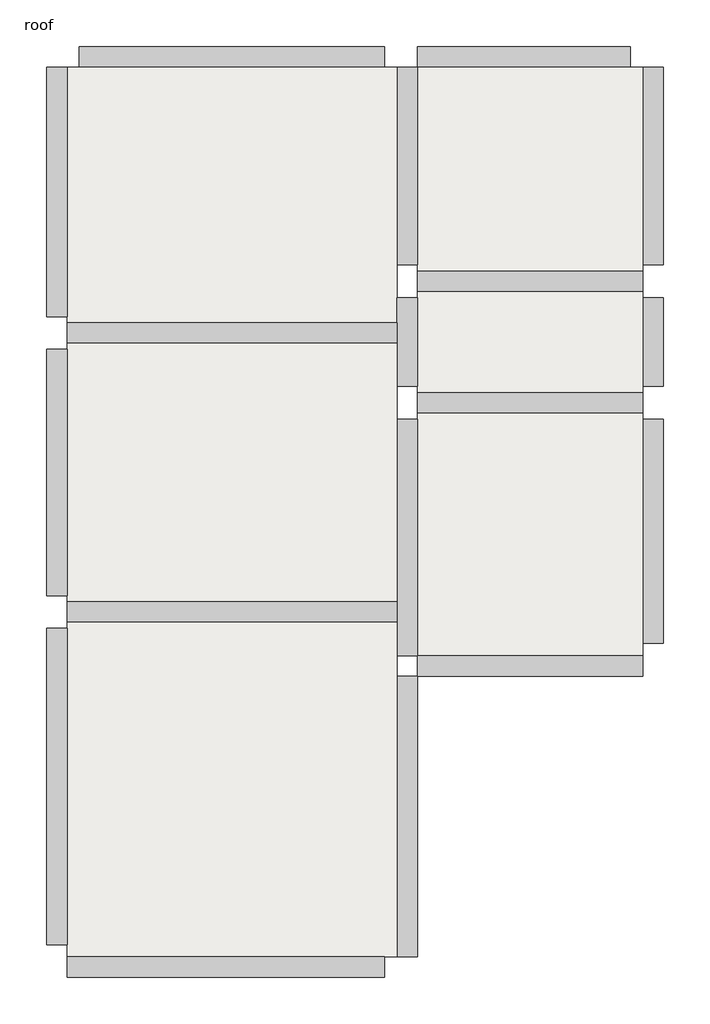
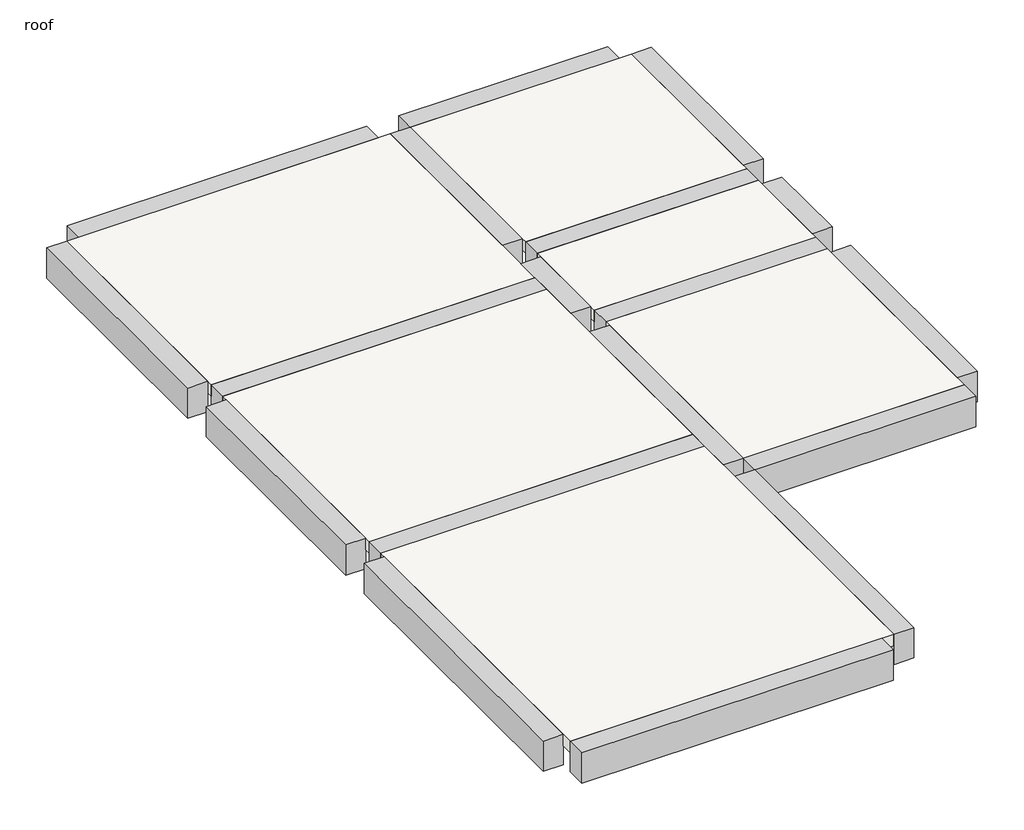
# One storey: 18 beams, 6 slabs.
"""IFC4 building model written with IfcOpenShell, lengths in millimetres."""

from ifc_helpers import new_model, si_unit, frame, origin, place, context, project, spatial, polyline, outline, extrude, faceted_brep, element, save

model = new_model("IFC4")

# Units and contexts
model_context = context("Model", 3, world=origin())
ifc_project = project(units=[si_unit("LENGTHUNIT", "METRE", prefix="MILLI")], contexts=[model_context])

# Site, building, storey
site = spatial("IfcSite", under=ifc_project)
building = spatial("IfcBuilding", under=site)
storey = spatial("IfcBuildingStorey", under=building, Name="roof", Elevation=6400.8)

# Beams
placement = place(None, origin())
element("IfcBeam", 1, ObjectType="Concrete-Rectangular Beam : BEAM", at=placement, inside=storey, context=model_context, shape_type="SweptSolid", body=[
    extrude(outline(polyline([(-12336.5990423, 3901.2699494), (-12082.5990423, 3901.2699494), (-12082.5990423, -16.6800506), (-12336.5990423, -16.6800506), (-12336.5990423, 3901.2699494)])), frame((0.0, 0.0, 5994.4), z_axis=(0.0, 0.0, 1.0), x_axis=(1.0, 0.0, 0.0)), (0.0, 0.0, 1.0), 406.4),
])
element("IfcBeam", 2, ObjectType="Concrete-Rectangular Beam : BEAM", at=placement, inside=storey, context=model_context, shape_type="SweptSolid", body=[
    extrude(outline(polyline([(-12336.5990423, 7355.6699494), (-12082.5990423, 7355.6699494), (-12082.5990423, 4307.6699494), (-12336.5990423, 4307.6699494), (-12336.5990423, 7355.6699494)])), frame((0.0, 0.0, 5994.4), z_axis=(0.0, 0.0, 1.0), x_axis=(1.0, 0.0, 0.0)), (0.0, 0.0, 1.0), 406.4),
])
element("IfcBeam", 3, ObjectType="Concrete-Rectangular Beam : BEAM", at=placement, inside=storey, context=model_context, shape_type="Brep", body=[
    faceted_brep([(-12082.5990423, 10854.5199494, 6400.8), (-12336.5990423, 10854.5199494, 6400.8), (-12336.5990423, 7762.0699494, 6400.8), (-12082.5990423, 7762.0699494, 6400.8), (-12082.5990423, 10854.5199494, 5994.4), (-12082.5990423, 10854.5199494, 6248.4), (-12082.5990423, 7762.0699494, 5994.4), (-12336.5990423, 10854.5199494, 5994.4), (-12336.5990423, 7762.0699494, 5994.4)], [[[0, 1, 2, 3]], [[4, 5, 0, 3, 6]], [[7, 4, 6, 8]], [[1, 7, 8, 2]], [[1, 0, 5, 4, 7]], [[3, 2, 8, 6]]]),
])
element("IfcBeam", 4, ObjectType="Concrete-Rectangular Beam : BEAM", at=placement, inside=storey, context=model_context, shape_type="SweptSolid", body=[
    extrude(outline(polyline([(-11930.1990423, 10854.5199494), (-11930.1990423, 11108.5199494), (-8145.5990423, 11108.5199494), (-8145.5990423, 10854.5199494), (-11930.1990423, 10854.5199494)])), frame((0.0, 0.0, 5994.4), z_axis=(0.0, 0.0, 1.0), x_axis=(1.0, 0.0, 0.0)), (0.0, 0.0, 1.0), 406.4),
])
element("IfcBeam", 5, ObjectType="Concrete-Rectangular Beam : BEAM", at=placement, inside=storey, context=model_context, shape_type="Brep", body=[
    faceted_brep([(-7739.1990423, 11108.5199494, 6400.8), (-7739.1990423, 10854.5199494, 6400.8), (-5097.5990423, 10854.5199494, 6400.8), (-5097.5990423, 11108.5199494, 6400.8), (-7739.1990423, 10854.5199494, 6248.4), (-7739.1990423, 10854.5199494, 5994.4), (-5097.5990423, 10854.5199494, 5994.4), (-7739.1990423, 11108.5199494, 5994.4), (-5097.5990423, 11108.5199494, 5994.4)], [[[0, 1, 2, 3]], [[1, 4, 5, 6, 2]], [[5, 7, 8, 6]], [[7, 0, 3, 8]], [[5, 4, 1, 0, 7]], [[3, 2, 6, 8]]]),
])
element("IfcBeam", 6, ObjectType="Concrete-Rectangular Beam : BEAM", at=placement, inside=storey, context=model_context, shape_type="Brep", body=[
    faceted_brep([(-4691.1990423, 10854.5199494, 6400.8), (-4945.1990423, 10854.5199494, 6400.8), (-4945.1990423, 8403.4199494, 6400.8), (-4691.1990423, 8403.4199494, 6400.8), (-4691.1990423, 10854.5199494, 5994.4), (-4691.1990423, 8403.4199494, 5994.4), (-4945.1990423, 10854.5199494, 5994.4), (-4945.1990423, 8403.4199494, 5994.4), (-4945.1990423, 10854.5199494, 6248.4)], [[[0, 1, 2, 3]], [[4, 0, 3, 5]], [[6, 4, 5, 7]], [[1, 8, 6, 7, 2]], [[6, 8, 1, 0, 4]], [[3, 2, 7, 5]]]),
])
element("IfcBeam", 7, ObjectType="Concrete-Rectangular Beam : BEAM", at=placement, inside=storey, context=model_context, shape_type="SweptSolid", body=[
    extrude(outline(polyline([(-4945.1990423, 7997.0199494), (-4691.1990423, 7997.0199494), (-4691.1990423, 6898.4699494), (-4945.1990423, 6898.4699494), (-4945.1990423, 7997.0199494)])), frame((0.0, 0.0, 5994.4), z_axis=(0.0, 0.0, 1.0), x_axis=(1.0, 0.0, 0.0)), (0.0, 0.0, 1.0), 406.4),
])
element("IfcBeam", 8, ObjectType="Concrete-Rectangular Beam : BEAM", at=placement, inside=storey, context=model_context, shape_type="SweptSolid", body=[
    extrude(outline(polyline([(-4691.1990423, 3717.1199494), (-4945.1990423, 3717.1199494), (-4945.1990423, 6492.0699494), (-4691.1990423, 6492.0699494), (-4691.1990423, 3717.1199494)])), frame((0.0, 0.0, 5994.4), z_axis=(0.0, 0.0, 1.0), x_axis=(1.0, 0.0, 0.0)), (0.0, 0.0, 1.0), 406.4),
])
element("IfcBeam", 9, ObjectType="Concrete-Rectangular Beam : BEAM", at=placement, inside=storey, context=model_context, shape_type="Brep", body=[
    faceted_brep([(-4945.1990423, 3310.7199494, 6400.8), (-4945.1990423, 3564.7199494, 6400.8), (-7739.1990423, 3564.7199494, 6400.8), (-7739.1990423, 3310.7199494, 6400.8), (-4945.1990423, 3564.7199494, 6248.4), (-4945.1990423, 3564.7199494, 5994.4), (-7739.1990423, 3564.7199494, 5994.4), (-7739.1990423, 3564.7199494, 6248.4), (-4945.1990423, 3310.7199494, 5994.4), (-7739.1990423, 3310.7199494, 5994.4)], [[[0, 1, 2, 3]], [[1, 4, 5, 6, 7, 2]], [[5, 8, 9, 6]], [[3, 9, 8, 0]], [[0, 8, 5, 4, 1]], [[3, 2, 7, 6, 9]]]),
])
element("IfcBeam", 10, ObjectType="Concrete-Rectangular Beam : BEAM", at=placement, inside=storey, context=model_context, shape_type="Brep", body=[
    faceted_brep([(-7993.1990423, 3564.7199494, 6400.8), (-7739.1990423, 3564.7199494, 6400.8), (-7739.1990423, 6492.0699494, 6400.8), (-7993.1990423, 6492.0699494, 6400.8), (-7993.1990423, 4231.4699494, 6400.8), (-7993.1990423, 3977.4699494, 6400.8), (-7993.1990423, 3564.7199494, 5994.4), (-7993.1990423, 6492.0699494, 5994.4), (-7993.1990423, 4231.4699494, 5994.4), (-7993.1990423, 3977.4699494, 5994.4), (-7739.1990423, 3564.7199494, 5994.4), (-7739.1990423, 6492.0699494, 5994.4), (-7739.1990423, 3564.7199494, 6248.4)], [[[0, 1, 2, 3, 4, 5]], [[6, 0, 5, 4, 3, 7, 8, 9]], [[10, 6, 9, 8, 7, 11]], [[1, 12, 10, 11, 2]], [[10, 12, 1, 0, 6]], [[3, 2, 11, 7]]]),
])
element("IfcBeam", 11, ObjectType="Concrete-Rectangular Beam : BEAM", at=placement, inside=storey, context=model_context, shape_type="Brep", body=[
    faceted_brep([(-7993.1990423, 6898.4699494, 6400.8), (-7739.1990423, 6898.4699494, 6400.8), (-7739.1990423, 7997.0199494, 6400.8), (-7993.1990423, 7997.0199494, 6400.8), (-7993.1990423, 7685.8699494, 6400.8), (-7993.1990423, 7431.8699494, 6400.8), (-7739.1990423, 6898.4699494, 5994.4), (-7739.1990423, 7997.0199494, 5994.4), (-7993.1990423, 6898.4699494, 5994.4), (-7993.1990423, 7431.8699494, 5994.4), (-7993.1990423, 7685.8699494, 5994.4), (-7993.1990423, 7997.0199494, 5994.4)], [[[0, 1, 2, 3, 4, 5]], [[1, 6, 7, 2]], [[6, 8, 9, 10, 11, 7]], [[8, 0, 5, 4, 3, 11, 10, 9]], [[1, 0, 8, 6]], [[3, 2, 7, 11]]]),
])
element("IfcBeam", 12, ObjectType="Concrete-Rectangular Beam : BEAM", at=placement, inside=storey, context=model_context, shape_type="Brep", body=[
    faceted_brep([(-7739.1990423, 10854.5199494, 6400.8), (-7993.1990423, 10854.5199494, 6400.8), (-7993.1990423, 8403.4199494, 6400.8), (-7739.1990423, 8403.4199494, 6400.8), (-7739.1990423, 10854.5199494, 5994.4), (-7739.1990423, 10854.5199494, 6248.4), (-7739.1990423, 8403.4199494, 5994.4), (-7993.1990423, 10854.5199494, 5994.4), (-7993.1990423, 8403.4199494, 5994.4), (-7993.1990423, 10854.5199494, 6248.4)], [[[0, 1, 2, 3]], [[4, 5, 0, 3, 6]], [[7, 4, 6, 8]], [[1, 9, 7, 8, 2]], [[7, 9, 1, 0, 5, 4]], [[3, 2, 8, 6]]]),
])
element("IfcBeam", 13, ObjectType="Concrete-Rectangular Beam : BEAM", at=placement, inside=storey, context=model_context, shape_type="Brep", body=[
    faceted_brep([(-7739.1990423, 3310.7199494, 6400.8), (-7993.1990423, 3310.7199494, 6400.8), (-7993.1990423, -169.0800506, 6400.8), (-7739.1990423, -169.0800506, 6400.8), (-7993.1990423, 3310.7199494, 5994.4), (-7993.1990423, -169.0800506, 5994.4), (-7993.1990423, -169.0800506, 6248.4), (-7739.1990423, 3310.7199494, 5994.4), (-7739.1990423, -169.0800506, 5994.4)], [[[0, 1, 2, 3]], [[1, 4, 5, 6, 2]], [[4, 7, 8, 5]], [[7, 0, 3, 8]], [[0, 7, 4, 1]], [[3, 2, 6, 5, 8]]]),
])
element("IfcBeam", 14, ObjectType="Concrete-Rectangular Beam : BEAM", at=placement, inside=storey, context=model_context, shape_type="Brep", body=[
    faceted_brep([(-12082.5990423, -169.0800506, 6400.8), (-12082.5990423, -423.0800506, 6400.8), (-8145.5990423, -423.0800506, 6400.8), (-8145.5990423, -169.0800506, 6400.8), (-12082.5990423, -169.0800506, 5994.4), (-12082.5990423, -169.0800506, 6248.4), (-8145.5990423, -169.0800506, 5994.4), (-12082.5990423, -423.0800506, 5994.4), (-8145.5990423, -423.0800506, 5994.4)], [[[0, 1, 2, 3]], [[4, 5, 0, 3, 6]], [[7, 4, 6, 8]], [[1, 7, 8, 2]], [[0, 5, 4, 7, 1]], [[3, 2, 8, 6]]]),
])
element("IfcBeam", 15, ObjectType="Concrete-Rectangular Beam : BEAM", at=placement, inside=storey, context=model_context, shape_type="Brep", body=[
    faceted_brep([(-12082.5990423, 7685.8699494, 6400.8), (-12082.5990423, 7431.8699494, 6400.8), (-7993.1990423, 7431.8699494, 6400.8), (-7993.1990423, 7685.8699494, 6400.8), (-12082.5990423, 7431.8699494, 6248.4), (-12082.5990423, 7431.8699494, 5994.4), (-7993.1990423, 7431.8699494, 5994.4), (-7993.1990423, 7431.8699494, 6248.4), (-12082.5990423, 7685.8699494, 5994.4), (-7993.1990423, 7685.8699494, 5994.4), (-7993.1990423, 7685.8699494, 6248.4), (-12082.5990423, 7685.8699494, 6248.4)], [[[0, 1, 2, 3]], [[1, 4, 5, 6, 7, 2]], [[5, 8, 9, 6]], [[3, 10, 9, 8, 11, 0]], [[0, 11, 8, 5, 4, 1]], [[3, 2, 7, 6, 9, 10]]]),
])
element("IfcBeam", 16, ObjectType="Concrete-Rectangular Beam : BEAM", at=placement, inside=storey, context=model_context, shape_type="Brep", body=[
    faceted_brep([(-7739.1990423, 8327.2199494, 6400.8), (-7739.1990423, 8073.2199494, 6400.8), (-4945.1990423, 8073.2199494, 6400.8), (-4945.1990423, 8327.2199494, 6400.8), (-7739.1990423, 8073.2199494, 6248.4), (-7739.1990423, 8073.2199494, 5994.4), (-4945.1990423, 8073.2199494, 5994.4), (-4945.1990423, 8073.2199494, 6248.4), (-7739.1990423, 8327.2199494, 5994.4), (-4945.1990423, 8327.2199494, 5994.4), (-4945.1990423, 8327.2199494, 6248.4), (-7739.1990423, 8327.2199494, 6248.4)], [[[0, 1, 2, 3]], [[1, 4, 5, 6, 7, 2]], [[5, 8, 9, 6]], [[3, 10, 9, 8, 11, 0]], [[9, 10, 3, 2, 7, 6]], [[0, 11, 8, 5, 4, 1]]]),
])
element("IfcBeam", 17, ObjectType="Concrete-Rectangular Beam : BEAM", at=placement, inside=storey, context=model_context, shape_type="Brep", body=[
    faceted_brep([(-4945.1990423, 6568.2699494, 6400.8), (-4945.1990423, 6822.2699494, 6400.8), (-7739.1990423, 6822.2699494, 6400.8), (-7739.1990423, 6568.2699494, 6400.8), (-7739.1990423, 6568.2699494, 6248.4), (-7739.1990423, 6568.2699494, 5994.4), (-4945.1990423, 6568.2699494, 5994.4), (-4945.1990423, 6568.2699494, 6248.4), (-4945.1990423, 6822.2699494, 5994.4), (-7739.1990423, 6822.2699494, 5994.4), (-4945.1990423, 6822.2699494, 6248.4), (-7739.1990423, 6822.2699494, 6248.4)], [[[0, 1, 2, 3]], [[3, 4, 5, 6, 7, 0]], [[8, 6, 5, 9]], [[1, 10, 8, 9, 11, 2]], [[5, 4, 3, 2, 11, 9]], [[0, 7, 6, 8, 10, 1]]]),
])
element("IfcBeam", 18, ObjectType="Concrete-Rectangular Beam : BEAM", at=placement, inside=storey, context=model_context, shape_type="Brep", body=[
    faceted_brep([(-12082.5990423, 4231.4699494, 6400.8), (-12082.5990423, 3977.4699494, 6400.8), (-7993.1990423, 3977.4699494, 6400.8), (-7993.1990423, 4231.4699494, 6400.8), (-12082.5990423, 3977.4699494, 6248.4), (-12082.5990423, 3977.4699494, 5994.4), (-7993.1990423, 3977.4699494, 5994.4), (-7993.1990423, 3977.4699494, 6248.4), (-12082.5990423, 4231.4699494, 5994.4), (-7993.1990423, 4231.4699494, 5994.4), (-7993.1990423, 4231.4699494, 6248.4), (-12082.5990423, 4231.4699494, 6248.4)], [[[0, 1, 2, 3]], [[1, 4, 5, 6, 7, 2]], [[5, 8, 9, 6]], [[3, 10, 9, 8, 11, 0]], [[0, 11, 8, 5, 4, 1]], [[3, 2, 7, 6, 9, 10]]]),
])

# Slabs
element("IfcSlab", 19, ObjectType="6\" Foundation Slab", at=placement, inside=storey, context=model_context, shape_type="Brep", body=[
    faceted_brep([(-7993.1990423, 10854.5199494, 6248.4), (-7993.1990423, 7685.8699494, 6248.4), (-12082.5990423, 7685.8699494, 6248.4), (-12082.5990423, 10854.5199494, 6248.4), (-7993.1990423, 10854.5199494, 6400.8), (-8145.5990423, 10854.5199494, 6400.8), (-11930.1990423, 10854.5199494, 6400.8), (-12082.5990423, 10854.5199494, 6400.8), (-12082.5990423, 7762.0699494, 6400.8), (-12082.5990423, 7685.8699494, 6400.8), (-7993.1990423, 7685.8699494, 6400.8), (-7993.1990423, 7997.0199494, 6400.8), (-7993.1990423, 8403.4199494, 6400.8)], [[[0, 1, 2, 3]], [[4, 5, 6, 7, 8, 9, 10, 11, 12]], [[1, 0, 4, 12, 11, 10]], [[2, 1, 10, 9]], [[3, 2, 9, 8, 7]], [[0, 3, 7, 6, 5, 4]]]),
])
element("IfcSlab", 20, ObjectType="6\" Foundation Slab", at=placement, inside=storey, context=model_context, shape_type="Brep", body=[
    faceted_brep([(-4945.1990423, 10854.5199494, 6248.4), (-4945.1990423, 8327.2199494, 6248.4), (-7739.1990423, 8327.2199494, 6248.4), (-7739.1990423, 10854.5199494, 6248.4), (-4945.1990423, 10854.5199494, 6400.8), (-5097.5990423, 10854.5199494, 6400.8), (-7739.1990423, 10854.5199494, 6400.8), (-7739.1990423, 8403.4199494, 6400.8), (-7739.1990423, 8327.2199494, 6400.8), (-4945.1990423, 8327.2199494, 6400.8), (-4945.1990423, 8403.4199494, 6400.8)], [[[0, 1, 2, 3]], [[4, 5, 6, 7, 8, 9, 10]], [[1, 0, 4, 10, 9]], [[2, 1, 9, 8]], [[3, 2, 8, 7, 6]], [[0, 3, 6, 5, 4]]]),
])
element("IfcSlab", 21, ObjectType="6\" Foundation Slab", at=placement, inside=storey, context=model_context, shape_type="Brep", body=[
    faceted_brep([(-7993.1990423, 7431.8699494, 6248.4), (-7993.1990423, 4231.4699494, 6248.4), (-12082.5990423, 4231.4699494, 6248.4), (-12082.5990423, 7431.8699494, 6248.4), (-7993.1990423, 7431.8699494, 6400.8), (-12082.5990423, 7431.8699494, 6400.8), (-12082.5990423, 7355.6699494, 6400.8), (-12082.5990423, 4307.6699494, 6400.8), (-12082.5990423, 4231.4699494, 6400.8), (-7993.1990423, 4231.4699494, 6400.8), (-7993.1990423, 6492.0699494, 6400.8), (-7993.1990423, 6898.4699494, 6400.8)], [[[0, 1, 2, 3]], [[4, 5, 6, 7, 8, 9, 10, 11]], [[1, 0, 4, 11, 10, 9]], [[2, 1, 9, 8]], [[3, 2, 8, 7, 6, 5]], [[0, 3, 5, 4]]]),
])
element("IfcSlab", 22, ObjectType="6\" Foundation Slab", at=placement, inside=storey, context=model_context, shape_type="Brep", body=[
    faceted_brep([(-4945.1990423, 6568.2699494, 6248.4), (-4945.1990423, 3564.7199494, 6248.4), (-7739.1990423, 3564.7199494, 6248.4), (-7739.1990423, 6568.2699494, 6248.4), (-4945.1990423, 6568.2699494, 6400.8), (-7739.1990423, 6568.2699494, 6400.8), (-7739.1990423, 6492.0699494, 6400.8), (-7739.1990423, 3564.7199494, 6400.8), (-4945.1990423, 3564.7199494, 6400.8), (-4945.1990423, 3717.1199494, 6400.8), (-4945.1990423, 6492.0699494, 6400.8)], [[[0, 1, 2, 3]], [[4, 5, 6, 7, 8, 9, 10]], [[1, 0, 4, 10, 9, 8]], [[2, 1, 8, 7]], [[3, 2, 7, 6, 5]], [[0, 3, 5, 4]]]),
])
element("IfcSlab", 23, ObjectType="6\" Foundation Slab", at=placement, inside=storey, context=model_context, shape_type="Brep", body=[
    faceted_brep([(-7993.1990423, 3977.4699494, 6248.4), (-7993.1990423, -169.0800506, 6248.4), (-12082.5990423, -169.0800506, 6248.4), (-12082.5990423, 3977.4699494, 6248.4), (-7993.1990423, 3977.4699494, 6400.8), (-12082.5990423, 3977.4699494, 6400.8), (-12082.5990423, 3901.2699494, 6400.8), (-12082.5990423, -16.6800506, 6400.8), (-12082.5990423, -169.0800506, 6400.8), (-8145.5990423, -169.0800506, 6400.8), (-7993.1990423, -169.0800506, 6400.8), (-7993.1990423, 3310.7199494, 6400.8), (-7993.1990423, 3564.7199494, 6400.8)], [[[0, 1, 2, 3]], [[4, 5, 6, 7, 8, 9, 10, 11, 12]], [[1, 0, 4, 12, 11, 10]], [[2, 1, 10, 9, 8]], [[3, 2, 8, 7, 6, 5]], [[0, 3, 5, 4]]]),
])
element("IfcSlab", 24, ObjectType="6\" Foundation Slab", at=placement, inside=storey, context=model_context, shape_type="Brep", body=[
    faceted_brep([(-4945.1990423, 8073.2199494, 6248.4), (-4945.1990423, 6822.2699494, 6248.4), (-7739.1990423, 6822.2699494, 6248.4), (-7739.1990423, 8073.2199494, 6248.4), (-4945.1990423, 8073.2199494, 6400.8), (-7739.1990423, 8073.2199494, 6400.8), (-7739.1990423, 7997.0199494, 6400.8), (-7739.1990423, 6898.4699494, 6400.8), (-7739.1990423, 6822.2699494, 6400.8), (-4945.1990423, 6822.2699494, 6400.8), (-4945.1990423, 6898.4699494, 6400.8), (-4945.1990423, 7997.0199494, 6400.8)], [[[0, 1, 2, 3]], [[4, 5, 6, 7, 8, 9, 10, 11]], [[1, 0, 4, 11, 10, 9]], [[2, 1, 9, 8]], [[3, 2, 8, 7, 6, 5]], [[0, 3, 5, 4]]]),
])

save(model, "model.ifc")

# Revit data of these elements
# Type "Concrete-Rectangular Beam : BEAM"
#   Assembly Code = "B10"
#   Length [instance default] = 1524 mm
#   b = 254 mm
#   h = 406.4 mm
#   Structural Material [instance default] = Concrete, Cast-in-Place gray
# Type "6\" Foundation Slab"
#   Layers, outside or top first: 152.4 mm "Concrete, Cast-in-Place gray" (function 1)
# Elements 1, 2, 3, 4, 5, 6, 7, 8, 9, 10, 11, 12, 13, 14, 15, 16, 17, 18 (IfcBeam, "Concrete-Rectangular Beam : BEAM")
#   Structural Material = Concrete, Cast-in-Place gray
#   Phase Created = New Construction
#   Materials on its faces: "Concrete, Cast-in-Place gray"
# Elements 19, 20, 21, 22, 23, 24 (IfcSlab, "6\" Foundation Slab")
#   Height Offset From Level = 0 mm
#   built-in parameter 1001954 = 1
#   Phase Created = New Construction
#   Materials on its faces: "Concrete, Cast-in-Place gray"
# Materials
#   "Concrete, Cast-in-Place gray": class "Concrete", colour RGB 192 192 192, transparency 0, Description = "Cast-in-place concrete", Cost = 0
